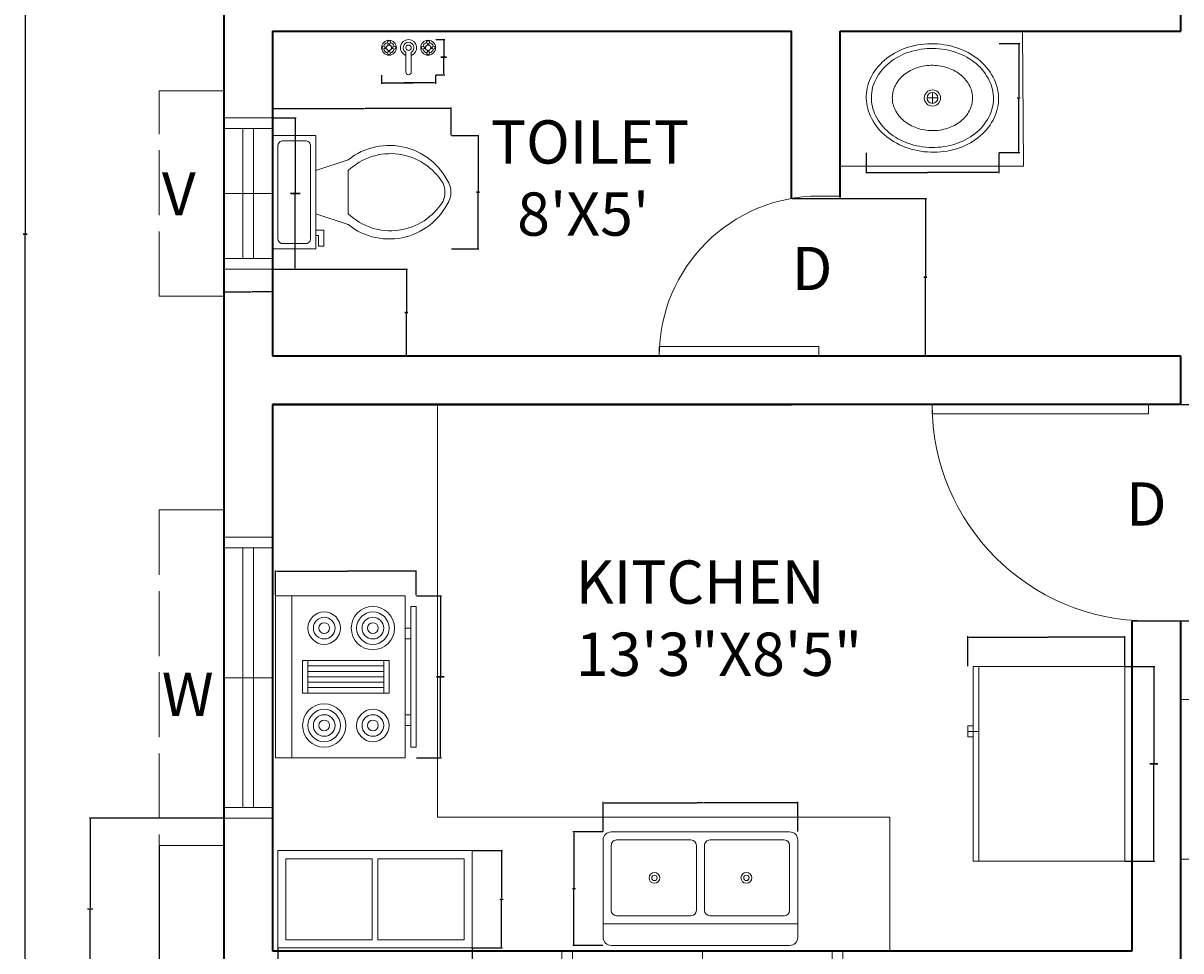
# Model space of a CAD drawing. Units: inches. Extents: x -35 to 832, y -515 to 219.
# Tile 3 of 7: x -35 to 179, y -163 to 9. Entities that reach past the tile are written whole.
import ezdxf

# ---------------------------------------------------------------- set-up
doc = ezdxf.new("R2010")
doc.units = ezdxf.units.IN
doc.header["$MEASUREMENT"] = 0
doc.linetypes.add('ACAD_ISO02W100', pattern=[15, 12, -3])
for name, color, linetype, lineweight in [('A-ANNO-TEXT', 7, 'Continuous', 18), ('A-AREA-IDEN', 7, 'Continuous', 18), ('A-DOOR', 4, 'Continuous', 18), ('A-EQPM', 8, 'Continuous', 18), ('A-FLOR-CASE', 3, 'Continuous', 18), ('A-FLOR-FIXT', 9, 'Continuous', 18), ('A-GLAZ', 2, 'Continuous', 18), ('A-GLAZ-OVHD', 2, 'ACAD_ISO02W100', 13), ('A-WALL', 10, 'Continuous', 35), ('S-ANNO-DIMS', 2, 'Continuous', 18)]:
    doc.layers.add(name, color=color, linetype=linetype, lineweight=lineweight)
doc.styles.get("Standard").update_dxf_attribs({"font": 'arial.ttf'})
doc.dimstyles.get("Standard").update_dxf_attribs({"dimtxt": 0.18, "dimasz": 0.18, "dimexe": 0.18, "dimexo": 0.0625, "dimgap": 0.09, "dimtad": 0, "dimtih": 1, "dimtoh": 1, "dimdec": 1, "dimzin": 0, "dimdsep": 46, "dimlunit": 4, "dimtxsty": 'Standard', "dimcen": 0.09, "dimclrd": 211, "dimclre": 4, "dimclrt": 3, "dimadec": 0, "dimazin": 0, "dimtfac": 0.5, "dimtdec": 1, "dimtofl": 0, "dimtmove": 0, "dimatfit": 3, "dimfxl": 1, "dimtfill": 2, "dimtfillclr": 61, "dimtolj": 1, "dimtzin": 0, "dimarcsym": 0})

# ---------------------------------------------------------------- blocks, each defined once
blk = doc.blocks.new('*U2')
for p, q in [((0, 0), (0, -6)), ((-40, 0), (-40, -6))]:
    blk.add_line(p, q)
blk.add_lwpolyline([(0, 0), (0, 40), (-1.75, 40), (-1.75, 0)], close=True)
blk.add_arc((0, 0), 40, 90, 180)
blk = doc.blocks.new('*U4')
for p, q in [((0, 0), (0, -100)), ((750, 0), (750, -100))]:
    blk.add_line(p, q)
blk.add_lwpolyline([(0, 0), (0, 750), (43.75, 750), (43.75, 0)], close=True)
blk.add_arc((0, 0), 750, 0, 90)
blk = doc.blocks.new('Range-Oven - 30 in top')
for p, q in [((0, -3), (30, -3)), ((12, -6), (18, -6)), ((13, -20), (13, -6)), ((14, -6), (14, -20)), ((15, -20), (15, -6)), ((16, -6), (16, -20)), ((17, -20), (17, -6)), ((18, -20), (12, -20)), ((6, -24), (6, -25)), ((8, -25), (8, -24)), ((22, -25), (22, -24)), ((24, -24), (24, -25))]:
    blk.add_line(p, q)
for points in [[(0, -24), (0, 0), (30, 0), (30, -24)], [(12, -21), (12, -5), (18, -5), (18, -21)], [(2, -26), (2, -25), (28, -25), (28, -26)]]:
    blk.add_lwpolyline(points, close=True)
for centre, radius in [((6, -9), 4), ((6, -9), 3), ((24, -9), 3), ((6, -9), 2), ((6, -9), 1), ((24, -9), 2), ((24, -9), 1), ((24, -18), 4), ((6, -18), 3), ((6, -18), 2), ((6, -18), 1), ((24, -18), 3), ((24, -18), 2), ((24, -18), 1)]:
    blk.add_circle(centre, radius)
blk = doc.blocks.new('Sink-double - 36 in top')
for p, q in [((-18, -4), (18, -4)), ((-0.75, -18.5), (-0.75, -6.5)), ((0.75, -6.5), (0.75, -18.5))]:
    blk.add_line(p, q)
for points in [[(-16.5, 0), (16.5, 0)], [(-18, -19.5), (-18, -1.5)], [(18, -1.5), (18, -19.5)], [(-15.5, -5.5), (-1.75, -5.5)], [(1.75, -5.5), (15.5, -5.5)], [(-16.5, -18.5), (-16.5, -6.5)], [(16.5, -6.5), (16.5, -18.5)], [(16.5, -21), (-16.5, -21)], [(-1.75, -19.5), (-15.5, -19.5)], [(15.5, -19.5), (1.75, -19.5)]]:
    blk.add_lwpolyline(points)
for centre, radius in [((-8.5, -12.5), 1), ((-8.5, -12.5), 0.5), ((8.5, -12.5), 1), ((8.5, -12.5), 0.5)]:
    blk.add_circle(centre, radius)
for centre, radius, start, end in [((-16.5, -1.5), 1.5, 90, 180), ((16.5, -1.5), 1.5, 0, 90), ((-15.5, -6.5), 1, 90, 180), ((-1.75, -6.5), 1, 0, 90), ((1.75, -6.5), 1, 90, 180), ((15.5, -6.5), 1, 0, 90), ((-15.5, -18.5), 1, 180, 270), ((-1.75, -18.5), 1, 270, 0), ((1.75, -18.5), 1, 180, 270), ((15.5, -18.5), 1, 270, 0), ((-16.5, -19.5), 1.5, 180, 270), ((16.5, -19.5), 1.5, 270, 0)]:
    blk.add_arc(centre, radius, start, end)
blk = doc.blocks.new('Refrigerator-2 door - 36 in top')
for p, q in [((0, -26.999999), (36, -26.999999)), ((12, -26.999999), (12, -28.999999)), ((11, -27.999999), (11, -28.999999)), ((11, -28.999999), (13, -28.999999)), ((13, -28.999999), (13, -27.999999))]:
    blk.add_line(p, q)
blk.add_lwpolyline([(0, -27.999999), (0, 0), (36, 0), (36, -27.999999)], close=True)
blk = doc.blocks.new('Wall Cabinet - 18 x 36 in front')
for p, q in [((17.5, -1.5), (17.5, -16.5)), ((18.5, -16.5), (18.5, -1.5))]:
    blk.add_line(p, q)
blk.add_lwpolyline([(0, -18), (0, 0), (36, 0), (36, -18)], close=True)
for points in [[(17.5, -16.5), (1.5, -16.5), (1.5, -1.5), (17.5, -1.5)], [(18.5, -1.5), (34.5, -1.5), (34.5, -16.5), (18.5, -16.5)]]:
    blk.add_lwpolyline(points)
blk = doc.blocks.new('Toilet - top')
for p, q in [((9.5, -6), (9.5, -2)), ((-10, -8.5), (-8, -8.5)), ((-10, -9.5), (-10, -8.5)), ((-8, -8.5), (-8, -8)), ((-7, -8), (-7, -9.5)), ((-4, -8), (-6, -14)), ((4, -8), (6, -14)), ((-7, -9.5), (-10, -9.5)), ((4, -14), (-4, -14))]:
    blk.add_line(p, q)
blk.add_lwpolyline([(10.5, -8), (10.5, 0), (-10.5, 0), (-10.5, -8)], close=True)
for points in [[(-9.5, -2), (-9.5, -6)], [(8.5, -1), (-8.5, -1)], [(-8.5, -7), (8.5, -7)]]:
    blk.add_lwpolyline(points)
for centre, radius, start, end in [((-8.62, -1.88), 0.884, 81.8699, 188.1301), ((8.62, -1.88), 0.884, 351.8699, 98.1301), ((-8.62, -6.12), 0.884, 171.8699, 278.1301), ((8.62, -6.12), 0.884, 261.8699, 8.1301), ((3.52, -21.58), 12.17, 141.4691, 247.9714), ((4.2, -21.82), 11.33, 136.3677, 238.9468), ((-3.52, -21.58), 12.17, 292.0284, 38.5307), ((-4.2, -21.82), 11.33, 301.053, 43.6321), ((0, -27.88), 4, 245.7318, 294.2682), ((0, -29), 4, 254.8605, 285.1395)]:
    blk.add_arc(centre, radius, start, end)
blk = doc.blocks.new('Sink - Oval top')
for p, q in [((-1, 0), (1, 0)), ((0, 1), (0, -1))]:
    blk.add_line(p, q)
for points in [[(-12.23, 0.39, 0.117634), (-11.46, -3.36, 0.104469), (-8.88, -6.8, 0.090016), (-5.08, -9.07, 0.08192), (-0.32, -10.02, 0.08192), (4.49, -9.38, 0.090016), (8.42, -7.36, 0.104469), (11.22, -4.09, 0.117634), (12.23, -0.39, 0.117634), (11.46, 3.36, 0.104469), (8.88, 6.8, 0.090016), (5.08, 9.07, 0.08192), (0.32, 10.02, 0.08192), (-4.49, 9.38, 0.090016), (-8.42, 7.36, 0.104469), (-11.22, 4.09, 0.117634)], [(-11.29, 0.16, 0.118622), (-10.52, -3.25, 0.104678), (-8.07, -6.36, 0.089562), (-4.54, -8.37, 0.081185), (-0.13, -9.15, 0.081185), (4.3, -8.49, 0.089562), (7.89, -6.58, 0.104678), (10.42, -3.55, 0.118622), (11.29, -0.16, 0.118622), (10.52, 3.25, 0.104678), (8.07, 6.36, 0.089562), (4.54, 8.37, 0.081185), (0.13, 9.15, 0.081185), (-4.3, 8.49, 0.089562), (-7.89, 6.58, 0.104678), (-10.42, 3.55, 0.118622)], [(-7.42, 0.08, 0.118283), (-6.91, -2.17, 0.104607), (-5.29, -4.21, 0.089718), (-2.97, -5.53, 0.081436), (-0.07, -6.04, 0.081436), (2.84, -5.59, 0.089718), (5.2, -4.33, 0.104607), (6.86, -2.32, 0.118283), (7.42, -0.08, 0.118283), (6.91, 2.17, 0.104607), (5.29, 4.21, 0.089718), (2.97, 5.53, 0.081436), (0.07, 6.04, 0.081436), (-2.84, 5.59, 0.089718), (-5.2, 4.33, 0.104607), (-6.86, 2.32, 0.118283)]]:
    blk.add_lwpolyline(points, format="xyb", close=True)
for radius in [1.5, 1]:
    blk.add_circle((0, 0), radius)
blk = doc.blocks.new('Faucet - Bathroom top')
for p, q in [((-4.107, 0.125), (-4.375, 0.125)), ((-3.75, 0.4788), (-3.75, 0.75)), ((-3.5, 0.482), (-3.5, 0.75)), ((-3.1461, 0.125), (-2.875, 0.125)), ((3.143, 0.125), (2.875, 0.125)), ((3.5, 0.4788), (3.5, 0.75)), ((3.75, 0.482), (3.75, 0.75)), ((4.1039, 0.125), (4.375, 0.125)), ((-4.1039, -0.125), (-4.375, -0.125)), ((-3.75, -0.4821), (-3.75, -0.75)), ((-3.5, -0.4789), (-3.5, -0.75)), ((-3.143, -0.125), (-2.875, -0.125)), ((-0.5, -0.8639), (-0.5, -4.5)), ((0.5, -4.5), (0.5, -0.8631)), ((3.1461, -0.125), (2.875, -0.125)), ((3.5, -0.4821), (3.5, -0.75)), ((3.75, -0.4789), (3.75, -0.75)), ((4.107, -0.125), (4.375, -0.125))]:
    blk.add_line(p, q)
for centre, radius in [((-3.625, 0), 1.375), ((-4.625, 0), 0.2795), ((-3.625, 0), 0.5), ((-3.625, 1), 0.2795), ((-2.625, 0), 0.2795), ((0, 0), 0.5), ((3.625, 0), 1.375), ((2.625, 0), 0.2795), ((3.625, 0), 0.5), ((3.625, 1), 0.2795), ((4.625, 0), 0.2795), ((-3.625, -1), 0.2795), ((3.625, -1), 0.2795)]:
    blk.add_circle(centre, radius)
for centre, radius, start, end in [((-3.625, 0), 1, 105.2407, 164.2093), ((-3.625, 0), 1, 16.44125, 74.07887), ((0, 0), 1.5, 289.6514, 250.3603), ((0, 0), 1, 300.3431, 239.7554), ((3.625, 0), 1, 106.12, 164.0884), ((3.625, 0), 1, 16.23422, 73.90469), ((-3.625, 0), 1, 196.2342, 253.9047), ((-3.625, 0), 1, 286.12, 344.0884), ((3.625, 0), 1, 196.4413, 254.0789), ((3.625, 0), 1, 285.2407, 344.2093), ((0, -4.5), 0.5, 180, 0)]:
    blk.add_arc(centre, radius, start, end)
blk = doc.blocks.new('WIN-48')
for p, q in [((0, 9), (0, 0)), ((2, 9), (2, 0)), ((26, 9), (26, 0)), ((50, 9), (50, 0)), ((52, 9), (52, 0)), ((2, 5.5), (50, 5.5)), ((2, 3.5), (50, 3.5))]:
    blk.add_line(p, q)
blk = doc.blocks.new('VENT-24')
for p, q in [((9, 28), (0, 28)), ((9, 26), (0, 26)), ((3.5, 26), (3.5, 2)), ((5.5, 26), (5.5, 2)), ((9, 14), (0, 14)), ((9, 2), (0, 2)), ((9, 0), (0, 0))]:
    blk.add_line(p, q)
blk = doc.blocks.new('WIN-48-HOOD')
for p, q in [((5, 12), (0, 12)), ((0, 12), (0, 0)), ((57, 12), (62, 12)), ((62, 12), (62, 0)), ((0, 0), (62, 0))]:
    blk.add_line(p, q)
blk = doc.blocks.new('VENT-24-HOOD')
for p, q in [((12, 38), (0, 38)), ((0, 0), (0, 38)), ((12, 33), (12, 38)), ((12, 5), (12, 0)), ((12, 0), (0, 0))]:
    blk.add_line(p, q)
blk = doc.blocks.new('*D65')
at = {"layer": 'Defpoints', "color": 0, "transparency": 16777216}
for p in [(10.8, -8.95), (15, -8.95), (10.8, -36.95)]:
    blk.add_point(p, dxfattribs=at)
at = {"layer": 'S-ANNO-DIMS', "color": 4, "lineweight": -2, "transparency": 16777216}
for p, q in [((10.86, -8.95), (15.18, -8.95)), ((10.86, -36.95), (15.18, -36.95))]:
    blk.add_line(p, q, dxfattribs=at)
at = {"layer": 'S-ANNO-DIMS', "color": 211, "lineweight": -2, "transparency": 16777216}
for p, q in [((15, -9.13), (15, -22.77)), ((15, -36.77), (15, -23.13))]:
    blk.add_line(p, q, dxfattribs=at)
at = {"layer": 'S-ANNO-DIMS', "color": 211, "transparency": 16777216}
for points in [[(14.97, -9.13), (15.03, -9.13), (15, -8.95)], [(14.97, -36.77), (15.03, -36.77), (15, -36.95)]]:
    blk.add_solid(points, dxfattribs=at)
at = {"layer": 'S-ANNO-DIMS', "color": 3, "transparency": 16777216, "insert": (15, -22.95), "char_height": 0.18, "attachment_point": 5, "bg_fill": 1, "box_fill_scale": 1.25, "bg_fill_color": 61, "bg_fill_transparency": 0}
blk.add_mtext('\\A1;VENT 2\'-4" TYP.', dxfattribs=at)
blk = doc.blocks.new('*D66')
at = {"layer": 'Defpoints', "color": 0, "transparency": 16777216}
for p in [(1.8, -36.95), (10.8, -36.95), (10.8, -41.15)]:
    blk.add_point(p, dxfattribs=at)
at = {"layer": 'S-ANNO-DIMS', "color": 4, "lineweight": -2, "transparency": 16777216}
for p, q in [((1.8, -37.01), (1.8, -41.33)), ((10.8, -37.01), (10.8, -41.33))]:
    blk.add_line(p, q, dxfattribs=at)
at = {"layer": 'S-ANNO-DIMS', "color": 211, "lineweight": -2, "transparency": 16777216}
for p, q in [((1.98, -41.15), (5.66, -41.15)), ((10.62, -41.15), (6.94, -41.15))]:
    blk.add_line(p, q, dxfattribs=at)
at = {"layer": 'S-ANNO-DIMS', "color": 211, "transparency": 16777216}
for points in [[(1.98, -41.12), (1.98, -41.18), (1.8, -41.15)], [(10.62, -41.12), (10.62, -41.18), (10.8, -41.15)]]:
    blk.add_solid(points, dxfattribs=at)
at = {"layer": 'S-ANNO-DIMS', "color": 3, "transparency": 16777216, "insert": (6.3, -41.15), "char_height": 0.18, "attachment_point": 5, "bg_fill": 1, "box_fill_scale": 1.25, "bg_fill_color": 61, "bg_fill_transparency": 0}
blk.add_mtext('\\A1;0\'-9" TYP.', dxfattribs=at)
blk = doc.blocks.new('*D75')
at = {"layer": 'Defpoints', "color": 0, "transparency": 16777216}
for p in [(37.35, -97.29), (41.85, -97.29), (37.35, -127.29)]:
    blk.add_point(p, dxfattribs=at)
at = {"layer": 'S-ANNO-DIMS', "color": 4, "lineweight": -2, "transparency": 16777216}
for p, q in [((37.41, -97.29), (42.03, -97.29)), ((37.41, -127.29), (42.03, -127.29))]:
    blk.add_line(p, q, dxfattribs=at)
at = {"layer": 'S-ANNO-DIMS', "color": 211, "lineweight": -2, "transparency": 16777216}
for p, q in [((41.85, -97.47), (41.85, -112.1)), ((41.85, -127.11), (41.85, -112.47))]:
    blk.add_line(p, q, dxfattribs=at)
at = {"layer": 'S-ANNO-DIMS', "color": 211, "transparency": 16777216}
for points in [[(41.82, -97.47), (41.88, -97.47), (41.85, -97.29)], [(41.82, -127.11), (41.88, -127.11), (41.85, -127.29)]]:
    blk.add_solid(points, dxfattribs=at)
at = {"layer": 'S-ANNO-DIMS', "color": 3, "transparency": 16777216, "insert": (41.85, -112.29), "char_height": 0.18, "attachment_point": 5, "bg_fill": 1, "box_fill_scale": 1.25, "bg_fill_color": 61, "bg_fill_transparency": 0}
blk.add_mtext('\\A1;RANGE 2\'-6"', dxfattribs=at)
blk = doc.blocks.new('*D76')
at = {"layer": 'Defpoints', "color": 0, "transparency": 16777216}
for p in [(11.35, -92.79), (11.35, -97.29), (37.35, -97.29)]:
    blk.add_point(p, dxfattribs=at)
at = {"layer": 'S-ANNO-DIMS', "color": 4, "lineweight": -2, "transparency": 16777216}
for p, q in [((11.35, -97.22), (11.35, -92.61)), ((37.35, -97.22), (37.35, -92.61))]:
    blk.add_line(p, q, dxfattribs=at)
at = {"layer": 'S-ANNO-DIMS', "color": 211, "lineweight": -2, "transparency": 16777216}
for p, q in [((11.53, -92.79), (24.02, -92.79)), ((37.17, -92.79), (24.68, -92.79))]:
    blk.add_line(p, q, dxfattribs=at)
at = {"layer": 'S-ANNO-DIMS', "color": 211, "transparency": 16777216}
for points in [[(11.53, -92.76), (11.53, -92.82), (11.35, -92.79)], [(37.17, -92.76), (37.17, -92.82), (37.35, -92.79)]]:
    blk.add_solid(points, dxfattribs=at)
at = {"layer": 'S-ANNO-DIMS', "color": 3, "transparency": 16777216, "insert": (24.35, -92.79), "char_height": 0.18, "attachment_point": 5, "bg_fill": 1, "box_fill_scale": 1.25, "bg_fill_color": 61, "bg_fill_transparency": 0}
blk.add_mtext('\\A1;2\'-2"', dxfattribs=at)
blk = doc.blocks.new('*D77')
at = {"layer": 'Defpoints', "color": 0, "transparency": 16777216}
for p in [(71.94, -135.56), (71.94, -140.96), (107.94, -140.96)]:
    blk.add_point(p, dxfattribs=at)
at = {"layer": 'S-ANNO-DIMS', "color": 4, "lineweight": -2, "transparency": 16777216}
for p, q in [((71.94, -140.9), (71.94, -135.38)), ((107.94, -140.9), (107.94, -135.38))]:
    blk.add_line(p, q, dxfattribs=at)
at = {"layer": 'S-ANNO-DIMS', "color": 211, "lineweight": -2, "transparency": 16777216}
for p, q in [((72.12, -135.56), (89.29, -135.56)), ((107.76, -135.56), (90.6, -135.56))]:
    blk.add_line(p, q, dxfattribs=at)
at = {"layer": 'S-ANNO-DIMS', "color": 211, "transparency": 16777216}
for points in [[(72.12, -135.53), (72.12, -135.59), (71.94, -135.56)], [(107.76, -135.53), (107.76, -135.59), (107.94, -135.56)]]:
    blk.add_solid(points, dxfattribs=at)
at = {"layer": 'S-ANNO-DIMS', "color": 3, "transparency": 16777216, "insert": (89.94, -135.56), "char_height": 0.18, "attachment_point": 5, "bg_fill": 1, "box_fill_scale": 1.25, "bg_fill_color": 61, "bg_fill_transparency": 0}
blk.add_mtext('\\A1;SINK 3\'-0"', dxfattribs=at)
blk = doc.blocks.new('*D78')
at = {"layer": 'Defpoints', "color": 0, "transparency": 16777216}
for p in [(71.94, -140.96), (66.54, -161.96), (71.94, -161.96)]:
    blk.add_point(p, dxfattribs=at)
at = {"layer": 'S-ANNO-DIMS', "color": 4, "lineweight": -2, "transparency": 16777216}
for p, q in [((71.88, -140.96), (66.36, -140.96)), ((71.88, -161.96), (66.36, -161.96))]:
    blk.add_line(p, q, dxfattribs=at)
at = {"layer": 'S-ANNO-DIMS', "color": 211, "lineweight": -2, "transparency": 16777216}
for p, q in [((66.54, -141.14), (66.54, -151.28)), ((66.54, -161.78), (66.54, -151.64))]:
    blk.add_line(p, q, dxfattribs=at)
at = {"layer": 'S-ANNO-DIMS', "color": 211, "transparency": 16777216}
for points in [[(66.51, -141.14), (66.57, -141.14), (66.54, -140.96)], [(66.51, -161.78), (66.57, -161.78), (66.54, -161.96)]]:
    blk.add_solid(points, dxfattribs=at)
at = {"layer": 'S-ANNO-DIMS', "color": 3, "transparency": 16777216, "insert": (66.54, -151.46), "char_height": 0.18, "attachment_point": 5, "bg_fill": 1, "box_fill_scale": 1.25, "bg_fill_color": 61, "bg_fill_transparency": 0}
blk.add_mtext('\\A1;1\'-9"', dxfattribs=at)
blk = doc.blocks.new('*D79')
at = {"layer": 'Defpoints', "color": 0, "transparency": 16777216}
for p in [(168.41, -110.38), (168.41, -146.38), (173.81, -146.38)]:
    blk.add_point(p, dxfattribs=at)
at = {"layer": 'S-ANNO-DIMS', "color": 4, "lineweight": -2, "transparency": 16777216}
for p, q in [((168.48, -110.38), (173.99, -110.38)), ((168.48, -146.38), (173.99, -146.38))]:
    blk.add_line(p, q, dxfattribs=at)
at = {"layer": 'S-ANNO-DIMS', "color": 211, "lineweight": -2, "transparency": 16777216}
for p, q in [((173.81, -110.56), (173.81, -128.19)), ((173.81, -146.2), (173.81, -128.56))]:
    blk.add_line(p, q, dxfattribs=at)
at = {"layer": 'S-ANNO-DIMS', "color": 211, "transparency": 16777216}
for points in [[(173.78, -110.56), (173.84, -110.56), (173.81, -110.38)], [(173.78, -146.2), (173.84, -146.2), (173.81, -146.38)]]:
    blk.add_solid(points, dxfattribs=at)
at = {"layer": 'S-ANNO-DIMS', "color": 3, "transparency": 16777216, "insert": (173.81, -128.38), "char_height": 0.18, "attachment_point": 5, "bg_fill": 1, "box_fill_scale": 1.25, "bg_fill_color": 61, "bg_fill_transparency": 0}
blk.add_mtext('\\A1;FRIDGE 3\'-0"', dxfattribs=at)
blk = doc.blocks.new('*D80')
at = {"layer": 'Defpoints', "color": 0, "transparency": 16777216}
for p in [(168.41, -104.98), (139.41, -110.38), (168.41, -110.38)]:
    blk.add_point(p, dxfattribs=at)
at = {"layer": 'S-ANNO-DIMS', "color": 4, "lineweight": -2, "transparency": 16777216}
for p, q in [((139.41, -110.31), (139.41, -104.8)), ((168.41, -110.31), (168.41, -104.8))]:
    blk.add_line(p, q, dxfattribs=at)
at = {"layer": 'S-ANNO-DIMS', "color": 211, "lineweight": -2, "transparency": 16777216}
for p, q in [((139.59, -104.98), (153.58, -104.98)), ((168.23, -104.98), (154.24, -104.98))]:
    blk.add_line(p, q, dxfattribs=at)
at = {"layer": 'S-ANNO-DIMS', "color": 211, "transparency": 16777216}
for points in [[(139.59, -104.95), (139.59, -105.01), (139.41, -104.98)], [(168.23, -104.95), (168.23, -105.01), (168.41, -104.98)]]:
    blk.add_solid(points, dxfattribs=at)
at = {"layer": 'S-ANNO-DIMS', "color": 3, "transparency": 16777216, "insert": (153.91, -104.98), "char_height": 0.18, "attachment_point": 5, "bg_fill": 1, "box_fill_scale": 1.25, "bg_fill_color": 61, "bg_fill_transparency": 0}
blk.add_mtext('\\A1;2\'-5"', dxfattribs=at)
blk = doc.blocks.new('*D81')
at = {"layer": 'Defpoints', "color": 0, "transparency": 16777216}
for p in [(11.74, -162.42), (47.74, -162.42), (47.74, -167.82)]:
    blk.add_point(p, dxfattribs=at)
at = {"layer": 'S-ANNO-DIMS', "color": 4, "lineweight": -2, "transparency": 16777216}
for p, q in [((11.74, -162.48), (11.74, -168)), ((47.74, -162.48), (47.74, -168))]:
    blk.add_line(p, q, dxfattribs=at)
at = {"layer": 'S-ANNO-DIMS', "color": 211, "lineweight": -2, "transparency": 16777216}
for p, q in [((11.92, -167.82), (28.83, -167.82)), ((47.56, -167.82), (30.65, -167.82))]:
    blk.add_line(p, q, dxfattribs=at)
at = {"layer": 'S-ANNO-DIMS', "color": 211, "transparency": 16777216}
for points in [[(11.92, -167.79), (11.92, -167.85), (11.74, -167.82)], [(47.56, -167.79), (47.56, -167.85), (47.74, -167.82)]]:
    blk.add_solid(points, dxfattribs=at)
at = {"layer": 'S-ANNO-DIMS', "color": 3, "transparency": 16777216, "insert": (29.74, -167.82), "char_height": 0.18, "attachment_point": 5, "bg_fill": 1, "box_fill_scale": 1.25, "bg_fill_color": 61, "bg_fill_transparency": 0}
blk.add_mtext('\\A1;CABINET 3\'-0"', dxfattribs=at)
blk = doc.blocks.new('*D82')
at = {"layer": 'Defpoints', "color": 0, "transparency": 16777216}
for p in [(47.74, -144.42), (53.14, -144.42), (47.74, -162.42)]:
    blk.add_point(p, dxfattribs=at)
at = {"layer": 'S-ANNO-DIMS', "color": 4, "lineweight": -2, "transparency": 16777216}
for p, q in [((47.8, -144.42), (53.32, -144.42)), ((47.8, -162.42), (53.32, -162.42))]:
    blk.add_line(p, q, dxfattribs=at)
at = {"layer": 'S-ANNO-DIMS', "color": 211, "lineweight": -2, "transparency": 16777216}
for p, q in [((53.14, -144.6), (53.14, -153.24)), ((53.14, -162.24), (53.14, -153.6))]:
    blk.add_line(p, q, dxfattribs=at)
at = {"layer": 'S-ANNO-DIMS', "color": 211, "transparency": 16777216}
for points in [[(53.11, -144.6), (53.17, -144.6), (53.14, -144.42)], [(53.11, -162.24), (53.17, -162.24), (53.14, -162.42)]]:
    blk.add_solid(points, dxfattribs=at)
at = {"layer": 'S-ANNO-DIMS', "color": 3, "transparency": 16777216, "insert": (53.14, -153.42), "char_height": 0.18, "attachment_point": 5, "bg_fill": 1, "box_fill_scale": 1.25, "bg_fill_color": 61, "bg_fill_transparency": 0}
blk.add_mtext('\\A1;1\'-6"', dxfattribs=at)
blk = doc.blocks.new('*D83')
at = {"layer": 'Defpoints', "color": 0, "transparency": 16777216}
for p in [(10.8, -7.24), (10.8, -12.2), (43.85, -12.2)]:
    blk.add_point(p, dxfattribs=at)
at = {"layer": 'S-ANNO-DIMS', "color": 4, "lineweight": -2, "transparency": 16777216}
for p, q in [((10.8, -12.13), (10.8, -7.06)), ((43.85, -12.13), (43.85, -7.06))]:
    blk.add_line(p, q, dxfattribs=at)
at = {"layer": 'S-ANNO-DIMS', "color": 211, "lineweight": -2, "transparency": 16777216}
for p, q in [((10.98, -7.24), (26.75, -7.24)), ((43.67, -7.24), (27.9, -7.24))]:
    blk.add_line(p, q, dxfattribs=at)
at = {"layer": 'S-ANNO-DIMS', "color": 211, "transparency": 16777216}
for points in [[(10.98, -7.21), (10.98, -7.27), (10.8, -7.24)], [(43.67, -7.21), (43.67, -7.27), (43.85, -7.24)]]:
    blk.add_solid(points, dxfattribs=at)
at = {"layer": 'S-ANNO-DIMS', "color": 3, "transparency": 16777216, "insert": (27.32, -7.24), "char_height": 0.18, "attachment_point": 5, "bg_fill": 1, "box_fill_scale": 1.25, "bg_fill_color": 61, "bg_fill_transparency": 0}
blk.add_mtext('\\A1;WC 2\'-9"', dxfattribs=at)
blk = doc.blocks.new('*D84')
at = {"layer": 'Defpoints', "color": 0, "transparency": 16777216}
for p in [(43.85, -12.2), (48.8, -12.2), (43.85, -33.2)]:
    blk.add_point(p, dxfattribs=at)
at = {"layer": 'S-ANNO-DIMS', "color": 4, "lineweight": -2, "transparency": 16777216}
for p, q in [((43.91, -12.2), (48.98, -12.2)), ((43.91, -33.2), (48.98, -33.2))]:
    blk.add_line(p, q, dxfattribs=at)
at = {"layer": 'S-ANNO-DIMS', "color": 211, "lineweight": -2, "transparency": 16777216}
for p, q in [((48.8, -12.38), (48.8, -22.51)), ((48.8, -33.02), (48.8, -22.88))]:
    blk.add_line(p, q, dxfattribs=at)
at = {"layer": 'S-ANNO-DIMS', "color": 211, "transparency": 16777216}
for points in [[(48.77, -12.38), (48.83, -12.38), (48.8, -12.2)], [(48.77, -33.02), (48.83, -33.02), (48.8, -33.2)]]:
    blk.add_solid(points, dxfattribs=at)
at = {"layer": 'S-ANNO-DIMS', "color": 3, "transparency": 16777216, "insert": (48.8, -22.7), "char_height": 0.18, "attachment_point": 5, "bg_fill": 1, "box_fill_scale": 1.25, "bg_fill_color": 61, "bg_fill_transparency": 0}
blk.add_mtext('\\A1;1\'-9"', dxfattribs=at)
blk = doc.blocks.new('*D85')
at = {"layer": 'Defpoints', "color": 0, "transparency": 16777216}
for p in [(120.58, -15.35), (145.13, -15.35), (145.13, -19.03)]:
    blk.add_point(p, dxfattribs=at)
at = {"layer": 'S-ANNO-DIMS', "color": 4, "lineweight": -2, "transparency": 16777216}
for p, q in [((120.58, -15.41), (120.58, -19.21)), ((145.13, -15.41), (145.13, -19.21))]:
    blk.add_line(p, q, dxfattribs=at)
at = {"layer": 'S-ANNO-DIMS', "color": 211, "lineweight": -2, "transparency": 16777216}
for p, q in [((120.76, -19.03), (131.91, -19.03)), ((144.95, -19.03), (133.8, -19.03))]:
    blk.add_line(p, q, dxfattribs=at)
at = {"layer": 'S-ANNO-DIMS', "color": 211, "transparency": 16777216}
for points in [[(120.76, -19), (120.76, -19.06), (120.58, -19.03)], [(144.95, -19), (144.95, -19.06), (145.13, -19.03)]]:
    blk.add_solid(points, dxfattribs=at)
at = {"layer": 'S-ANNO-DIMS', "color": 3, "transparency": 16777216, "insert": (132.85, -19.03), "char_height": 0.18, "attachment_point": 5, "bg_fill": 1, "box_fill_scale": 1.25, "bg_fill_color": 61, "bg_fill_transparency": 0}
blk.add_mtext('\\A1;BASIN 2\'-0 1/2"', dxfattribs=at)
blk = doc.blocks.new('*D86')
at = {"layer": 'Defpoints', "color": 0, "transparency": 16777216}
for p in [(145.13, 4.79), (148.81, 4.79), (145.13, -15.35)]:
    blk.add_point(p, dxfattribs=at)
at = {"layer": 'S-ANNO-DIMS', "color": 4, "lineweight": -2, "transparency": 16777216}
for p, q in [((145.19, 4.79), (148.99, 4.79)), ((145.19, -15.35), (148.99, -15.35))]:
    blk.add_line(p, q, dxfattribs=at)
at = {"layer": 'S-ANNO-DIMS', "color": 211, "lineweight": -2, "transparency": 16777216}
for p, q in [((148.81, 4.61), (148.81, -5.1)), ((148.81, -15.17), (148.81, -5.46))]:
    blk.add_line(p, q, dxfattribs=at)
at = {"layer": 'S-ANNO-DIMS', "color": 211, "transparency": 16777216}
for points in [[(148.78, 4.61), (148.84, 4.61), (148.81, 4.79)], [(148.78, -15.17), (148.84, -15.17), (148.81, -15.35)]]:
    blk.add_solid(points, dxfattribs=at)
at = {"layer": 'S-ANNO-DIMS', "color": 3, "transparency": 16777216, "insert": (148.81, -5.28), "char_height": 0.18, "attachment_point": 5, "bg_fill": 1, "box_fill_scale": 1.25, "bg_fill_color": 61, "bg_fill_transparency": 0}
blk.add_mtext('\\A1;1\'-8"', dxfattribs=at)
blk = doc.blocks.new('*D87')
at = {"layer": 'Defpoints', "color": 0, "transparency": 16777216}
for p in [(30.95, -0.99), (40.95, -0.99), (40.95, -2.49)]:
    blk.add_point(p, dxfattribs=at)
at = {"layer": 'S-ANNO-DIMS', "color": 4, "lineweight": -2, "transparency": 16777216}
for p, q in [((30.95, -1.05), (30.95, -2.67)), ((40.95, -1.05), (40.95, -2.67))]:
    blk.add_line(p, q, dxfattribs=at)
at = {"layer": 'S-ANNO-DIMS', "color": 211, "lineweight": -2, "transparency": 16777216}
for p, q in [((31.13, -2.49), (35.02, -2.49)), ((40.77, -2.49), (36.88, -2.49))]:
    blk.add_line(p, q, dxfattribs=at)
at = {"layer": 'S-ANNO-DIMS', "color": 211, "transparency": 16777216}
for points in [[(31.13, -2.46), (31.13, -2.52), (30.95, -2.49)], [(40.77, -2.46), (40.77, -2.52), (40.95, -2.49)]]:
    blk.add_solid(points, dxfattribs=at)
at = {"layer": 'S-ANNO-DIMS', "color": 3, "transparency": 16777216, "insert": (35.95, -2.49), "char_height": 0.18, "attachment_point": 5, "bg_fill": 1, "box_fill_scale": 1.25, "bg_fill_color": 61, "bg_fill_transparency": 0}
blk.add_mtext('\\A1;FAUCET 0\'-10"', dxfattribs=at)
blk = doc.blocks.new('*D88')
at = {"layer": 'Defpoints', "color": 0, "transparency": 16777216}
for p in [(40.95, 5.51), (42.45, 5.51), (40.95, -0.99)]:
    blk.add_point(p, dxfattribs=at)
at = {"layer": 'S-ANNO-DIMS', "color": 4, "lineweight": -2, "transparency": 16777216}
for p, q in [((41.02, 5.51), (42.63, 5.51)), ((41.02, -0.99), (42.63, -0.99))]:
    blk.add_line(p, q, dxfattribs=at)
at = {"layer": 'S-ANNO-DIMS', "color": 211, "lineweight": -2, "transparency": 16777216}
for p, q in [((42.45, 5.33), (42.45, 2.44)), ((42.45, -0.81), (42.45, 2.07))]:
    blk.add_line(p, q, dxfattribs=at)
at = {"layer": 'S-ANNO-DIMS', "color": 211, "transparency": 16777216}
for points in [[(42.42, 5.33), (42.48, 5.33), (42.45, 5.51)], [(42.42, -0.81), (42.48, -0.81), (42.45, -0.99)]]:
    blk.add_solid(points, dxfattribs=at)
at = {"layer": 'S-ANNO-DIMS', "color": 3, "transparency": 16777216, "insert": (42.45, 2.26), "char_height": 0.18, "attachment_point": 5, "bg_fill": 1, "box_fill_scale": 1.25, "bg_fill_color": 61, "bg_fill_transparency": 0}
blk.add_mtext('\\A1;0\'-6 1/2"', dxfattribs=at)
blk = doc.blocks.new('*D109')
at = {"layer": 'Defpoints', "color": 0, "transparency": 16777216}
for p in [(365.8, -100.95), (-10.2, -143.45), (365.8, -279.7)]:
    blk.add_point(p, dxfattribs=at)
at = {"layer": 'S-ANNO-DIMS', "color": 4, "lineweight": -2, "transparency": 16777216}
for p, q in [((365.8, -101.01), (365.8, -279.88)), ((-10.2, -143.51), (-10.2, -279.88))]:
    blk.add_line(p, q, dxfattribs=at)
at = {"layer": 'S-ANNO-DIMS', "color": 211, "lineweight": -2, "transparency": 16777216}
for p, q in [((-10.02, -279.7), (177.4, -279.7)), ((365.62, -279.7), (178.2, -279.7))]:
    blk.add_line(p, q, dxfattribs=at)
at = {"layer": 'S-ANNO-DIMS', "color": 211, "transparency": 16777216}
for points in [[(-10.02, -279.67), (-10.02, -279.73), (-10.2, -279.7)], [(365.62, -279.67), (365.62, -279.73), (365.8, -279.7)]]:
    blk.add_solid(points, dxfattribs=at)
at = {"layer": 'S-ANNO-DIMS', "color": 3, "transparency": 16777216, "insert": (177.8, -279.7), "char_height": 0.18, "attachment_point": 5, "bg_fill": 1, "box_fill_scale": 1.25, "bg_fill_color": 61, "bg_fill_transparency": 0}
blk.add_mtext('\\A1;31\'-4"', dxfattribs=at)
blk = doc.blocks.new('*D110')
at = {"layer": 'Defpoints', "color": 0, "transparency": 16777216}
for p in [(59.3, 194.05), (-34.95, -254.95), (129.8, -254.95)]:
    blk.add_point(p, dxfattribs=at)
at = {"layer": 'S-ANNO-DIMS', "color": 4, "lineweight": -2, "transparency": 16777216}
for p, q in [((59.24, 194.05), (-35.13, 194.05)), ((129.74, -254.95), (-35.13, -254.95))]:
    blk.add_line(p, q, dxfattribs=at)
at = {"layer": 'S-ANNO-DIMS', "color": 211, "lineweight": -2, "transparency": 16777216}
for p, q in [((-34.95, 193.87), (-34.95, -30.27)), ((-34.95, -254.77), (-34.95, -30.63))]:
    blk.add_line(p, q, dxfattribs=at)
at = {"layer": 'S-ANNO-DIMS', "color": 211, "transparency": 16777216}
for points in [[(-34.98, 193.87), (-34.92, 193.87), (-34.95, 194.05)], [(-34.98, -254.77), (-34.92, -254.77), (-34.95, -254.95)]]:
    blk.add_solid(points, dxfattribs=at)
at = {"layer": 'S-ANNO-DIMS', "color": 3, "transparency": 16777216, "insert": (-34.95, -30.45), "char_height": 0.18, "attachment_point": 5, "bg_fill": 1, "box_fill_scale": 1.25, "bg_fill_color": 61, "bg_fill_transparency": 0}
blk.add_mtext('\\A1;37\'-5"', dxfattribs=at)
blk = doc.blocks.new('*D113')
at = {"layer": 'Defpoints', "color": 0, "transparency": 16777216}
for p in [(106.8, -23.86), (106.8, -52.95), (131.55, -52.95)]:
    blk.add_point(p, dxfattribs=at)
at = {"layer": 'S-ANNO-DIMS', "color": 4, "lineweight": -2, "transparency": 16777216}
for p, q in [((106.86, -23.86), (131.73, -23.86)), ((106.86, -52.95), (131.73, -52.95))]:
    blk.add_line(p, q, dxfattribs=at)
at = {"layer": 'S-ANNO-DIMS', "color": 211, "lineweight": -2, "transparency": 16777216}
for p, q in [((131.55, -24.04), (131.55, -38.22)), ((131.55, -52.77), (131.55, -38.59))]:
    blk.add_line(p, q, dxfattribs=at)
at = {"layer": 'S-ANNO-DIMS', "color": 211, "transparency": 16777216}
for points in [[(131.52, -24.04), (131.58, -24.04), (131.55, -23.86)], [(131.52, -52.77), (131.58, -52.77), (131.55, -52.95)]]:
    blk.add_solid(points, dxfattribs=at)
at = {"layer": 'S-ANNO-DIMS', "color": 3, "transparency": 16777216, "insert": (131.55, -38.41), "char_height": 0.18, "attachment_point": 5, "bg_fill": 1, "box_fill_scale": 1.25, "bg_fill_color": 61, "bg_fill_transparency": 0}
blk.add_mtext('\\A1;2\'-5"', dxfattribs=at)
blk = doc.blocks.new('*D114')
at = {"layer": 'Defpoints', "color": 0, "transparency": 16777216}
for p in [(169.8, -61.95), (169.8, -101.95), (194.55, -101.95)]:
    blk.add_point(p, dxfattribs=at)
at = {"layer": 'S-ANNO-DIMS', "color": 4, "lineweight": -2, "transparency": 16777216}
for p, q in [((169.86, -61.95), (194.73, -61.95)), ((169.86, -101.95), (194.73, -101.95))]:
    blk.add_line(p, q, dxfattribs=at)
at = {"layer": 'S-ANNO-DIMS', "color": 211, "lineweight": -2, "transparency": 16777216}
for p, q in [((194.55, -62.13), (194.55, -81.77)), ((194.55, -101.77), (194.55, -82.13))]:
    blk.add_line(p, q, dxfattribs=at)
at = {"layer": 'S-ANNO-DIMS', "color": 211, "transparency": 16777216}
for points in [[(194.52, -62.13), (194.58, -62.13), (194.55, -61.95)], [(194.52, -101.77), (194.58, -101.77), (194.55, -101.95)]]:
    blk.add_solid(points, dxfattribs=at)
at = {"layer": 'S-ANNO-DIMS', "color": 3, "transparency": 16777216, "insert": (194.55, -81.95), "char_height": 0.18, "attachment_point": 5, "bg_fill": 1, "box_fill_scale": 1.25, "bg_fill_color": 61, "bg_fill_transparency": 0}
blk.add_mtext('\\A1;3\'-4"', dxfattribs=at)
blk = doc.blocks.new('*D116')
at = {"layer": 'Defpoints', "color": 0, "transparency": 16777216}
for p in [(-22.95, -138.45), (1.8, -138.45), (1.8, -171.95)]:
    blk.add_point(p, dxfattribs=at)
at = {"layer": 'S-ANNO-DIMS', "color": 4, "lineweight": -2, "transparency": 16777216}
for p, q in [((1.74, -138.45), (-23.13, -138.45)), ((1.74, -171.95), (-23.13, -171.95))]:
    blk.add_line(p, q, dxfattribs=at)
at = {"layer": 'S-ANNO-DIMS', "color": 211, "lineweight": -2, "transparency": 16777216}
for p, q in [((-22.95, -138.63), (-22.95, -155.02)), ((-22.95, -171.77), (-22.95, -155.38))]:
    blk.add_line(p, q, dxfattribs=at)
at = {"layer": 'S-ANNO-DIMS', "color": 211, "transparency": 16777216}
for points in [[(-22.98, -138.63), (-22.92, -138.63), (-22.95, -138.45)], [(-22.98, -171.77), (-22.92, -171.77), (-22.95, -171.95)]]:
    blk.add_solid(points, dxfattribs=at)
at = {"layer": 'S-ANNO-DIMS', "color": 3, "transparency": 16777216, "insert": (-22.95, -155.2), "char_height": 0.18, "attachment_point": 5, "bg_fill": 1, "box_fill_scale": 1.25, "bg_fill_color": 61, "bg_fill_transparency": 0}
blk.add_mtext('\\A1;2\'-9 1/2"', dxfattribs=at)
blk = doc.blocks.new('*D117')
at = {"layer": 'Defpoints', "color": 0, "transparency": 16777216}
for p in [(10.8, -36.95), (10.8, -52.95), (35.55, -52.95)]:
    blk.add_point(p, dxfattribs=at)
at = {"layer": 'S-ANNO-DIMS', "color": 4, "lineweight": -2, "transparency": 16777216}
for p, q in [((10.86, -36.95), (35.73, -36.95)), ((10.86, -52.95), (35.73, -52.95))]:
    blk.add_line(p, q, dxfattribs=at)
at = {"layer": 'S-ANNO-DIMS', "color": 211, "lineweight": -2, "transparency": 16777216}
for p, q in [((35.55, -37.13), (35.55, -44.77)), ((35.55, -52.77), (35.55, -45.13))]:
    blk.add_line(p, q, dxfattribs=at)
at = {"layer": 'S-ANNO-DIMS', "color": 211, "transparency": 16777216}
for points in [[(35.52, -37.13), (35.58, -37.13), (35.55, -36.95)], [(35.52, -52.77), (35.58, -52.77), (35.55, -52.95)]]:
    blk.add_solid(points, dxfattribs=at)
at = {"layer": 'S-ANNO-DIMS', "color": 3, "transparency": 16777216, "insert": (35.55, -44.95), "char_height": 0.18, "attachment_point": 5, "bg_fill": 1, "box_fill_scale": 1.25, "bg_fill_color": 61, "bg_fill_transparency": 0}
blk.add_mtext('\\A1;1\'-4"', dxfattribs=at)

msp = doc.modelspace()

# ---------------------------------------------------------------- linework, layer by layer
at = {"layer": 'A-FLOR-CASE'}
for p, q in [((149.69, -17.88), (149.5, 7.05)), ((115.8, -17.88), (149.69, -17.88)), ((41.33, -61.95), (41.33, -138.22)), ((41.33, -138.22), (124.99, -138.22)), ((124.99, -138.22), (124.99, -162.95))]:
    msp.add_line(p, q, dxfattribs=at)
at = {"layer": 'A-WALL'}
for p, q in [((1.8, 182.05), (1.8, 7.05)), ((178.8, 7.05), (178.8, 16.05)), ((1.8, 7.05), (1.8, -52.95)), ((10.8, 7.05), (106.8, 7.05)), ((10.8, 7.05), (10.8, -52.95)), ((106.8, -23.86), (106.8, 7.05)), ((115.8, 7.05), (178.8, 7.05)), ((115.8, -23.69), (115.8, 7.05)), ((1.8, -52.95), (1.8, -171.95)), ((10.8, -52.95), (106.8, -52.95)), ((106.8, -52.95), (115.8, -52.95)), ((115.8, -52.95), (178.8, -52.95)), ((178.8, -61.95), (178.8, -52.95)), ((10.8, -61.95), (106.8, -61.95)), ((10.8, -61.95), (10.8, -162.95)), ((178.8, -61.95), (10.8, -61.95)), ((169.8, -62.06), (169.8, -61.95)), ((169.8, -162.95), (169.8, -101.95)), ((178.8, -171.95), (178.8, -101.95)), ((10.8, -162.95), (169.8, -162.95))]:
    msp.add_line(p, q, dxfattribs=at)

# ---------------------------------------------------------------- block references
at = {"layer": 'A-DOOR', "xscale": 0.0393700787401575, "yscale": 0.0393700787401575, "zscale": 0.0393700787401575, "rotation": 90}
msp.add_blockref('*U4', (111.86, -52.95), dxfattribs=at)
at = {"layer": 'A-DOOR', "rotation": 90}
msp.add_blockref('*U2', (172.8, -61.95), dxfattribs=at)
at = {"layer": 'A-DOOR', "xscale": 0.0393700787401575, "yscale": 0.0393700787401575, "zscale": 0.0393700787401575}
msp.add_blockref('*U4', (178.8, -146.01), dxfattribs=at)
at = {"layer": 'A-EQPM'}
for name, p, rotation in [('Range-Oven - 30 in top', (11.35, -127.29), 90), ('Refrigerator-2 door - 36 in top', (168.41, -110.38), 270)]:
    msp.add_blockref(name, p, dxfattribs=dict(at, rotation=rotation))
at = {"layer": 'A-FLOR-CASE'}
msp.add_blockref('Wall Cabinet - 18 x 36 in front', (11.74, -144.42), dxfattribs=at)
at = {"layer": 'A-FLOR-FIXT'}
for name, p in [('Faucet - Bathroom top', (35.95, 4.01)), ('Sink - Oval top', (132.85, -5.28))]:
    msp.add_blockref(name, p, dxfattribs=at)
for name, p, rotation in [('Toilet - top', (10.8, -22.7), 90), ('Sink-double - 36 in top', (89.94, -161.96), 180)]:
    msp.add_blockref(name, p, dxfattribs=dict(at, rotation=rotation))
at = {"layer": 'A-GLAZ'}
for name, p in [('VENT-24', (1.8, -36.95)), ('WIN-48', (64.3, -171.95))]:
    msp.add_blockref(name, p, dxfattribs=at)
at = {"layer": 'A-GLAZ', "rotation": 90.00000000000003}
msp.add_blockref('WIN-48', (10.8, -138.45), dxfattribs=at)
at = {"layer": 'A-GLAZ-OVHD'}
msp.add_blockref('VENT-24-HOOD', (-10.2, -41.95), dxfattribs=at)
at = {"layer": 'A-GLAZ-OVHD', "rotation": 270}
msp.add_blockref('WIN-48-HOOD', (-10.2, -81.45), dxfattribs=at)

# ---------------------------------------------------------------- texts
at = {"layer": 'A-ANNO-TEXT'}
for s, p in [('V', (-9.69, -27)), ('D', (106.84, -40.81)), ('D', (168.65, -84.34)), ('W', (-9.69, -119.52))]:
    msp.add_text(s, height=8, dxfattribs=at).set_placement(p)
at = {"layer": 'A-AREA-IDEN', "char_height": 8, "attachment_point": 1}
for s, insert in [("TOILET\\P  8'X5'", (51.15, -9.41)), ('KITCHEN\\P13\'3"X8\'5"', (66.87, -90.78))]:
    msp.add_mtext_dynamic_manual_height_columns(s, width=50.3004, gutter_width=1, heights=[0], dxfattribs=dict(at, insert=insert))

# ---------------------------------------------------------------- dimensions: what is measured, and where the dimension line sits
at = {"layer": 'S-ANNO-DIMS'}
for base, p1, p2, angle, picture, middle in [((-34.95, -254.95), (59.3, 194.05), (129.8, -254.95), 90, '*D110', (-34.95, -30.45)), ((42.45, 5.51), (40.95, -0.99), (40.95, 5.51), 90, '*D88', (42.45, 2.26)), ((148.81, 4.79), (145.13, -15.35), (145.13, 4.79), 90, '*D86', (148.81, -5.28)), ((48.8, -12.2), (43.85, -33.2), (43.85, -12.2), 90, '*D84', (48.8, -22.7)), ((131.55, -52.95), (106.8, -23.86), (106.8, -52.95), 270, '*D113', (131.55, -38.41)), ((35.55, -52.95), (10.8, -36.95), (10.8, -52.95), 270, '*D117', (35.55, -44.95)), ((194.55, -101.95), (169.8, -61.95), (169.8, -101.95), 270, '*D114', (194.55, -81.95)), ((11.35, -92.79), (37.35, -97.29), (11.35, -97.29), 180, '*D76', (24.35, -92.79)), ((-22.95, -138.45), (1.8, -171.95), (1.8, -138.45), 90, '*D116', (-22.95, -155.2)), ((66.54, -161.96), (71.94, -140.96), (71.94, -161.96), 270, '*D78', (66.54, -151.46)), ((53.14, -144.42), (47.74, -162.42), (47.74, -144.42), 90, '*D82', (53.14, -153.42))]:
    dim = msp.add_linear_dim(base=base, p1=p1, p2=p2, angle=angle, dimstyle='Standard', override={"dimdec": 1, "dimlfac": 1, "dimrnd": 0, "dimzin": 1, "dimdsep": 46, "dimlunit": 4, "dimfrac": 2}, dxfattribs=at)
    dim.commit()
    dim.dimension.update_dxf_attribs({"geometry": picture, "text_midpoint": middle})
for base, p1, p2, text, picture, middle in [((40.95, -2.49), (30.95, -0.99), (40.95, -0.99), 'FAUCET <>', '*D87', (35.95, -2.49)), ((145.1293, -19.0334), (120.5784, -15.3507), (145.1293, -15.3507), 'BASIN <>', '*D85', (132.8538, -19.0334)), ((10.8, -41.15), (1.8, -36.95), (10.8, -36.95), '<> TYP.', '*D66', (6.3, -41.15)), ((47.74, -167.82), (11.74, -162.42), (47.74, -162.42), 'CABINET <>', '*D81', (29.74, -167.82))]:
    dim = msp.add_linear_dim(base=base, p1=p1, p2=p2, text=text, dimstyle='Standard', override={"dimdec": 1, "dimlfac": 1, "dimrnd": 0, "dimzin": 1, "dimdsep": 46, "dimlunit": 4, "dimfrac": 2}, dxfattribs=at)
    dim.commit()
    dim.dimension.update_dxf_attribs({"geometry": picture, "text_midpoint": middle})
for base, p1, p2, angle, text, picture, middle in [((10.8006, -7.2397), (43.8469, -12.1967), (10.8006, -12.1967), 180, 'WC <>', '*D83', (27.3238, -7.2397)), ((15, -8.95), (10.8, -36.95), (10.8, -8.95), 90, 'VENT <> TYP.', '*D65', (15, -22.95)), ((41.85, -97.29), (37.35, -127.29), (37.35, -97.29), 90, 'RANGE <>', '*D75', (41.85, -112.29)), ((173.81, -146.38), (168.41, -110.38), (168.41, -146.38), 270, 'FRIDGE <>', '*D79', (173.81, -128.38)), ((71.94, -135.56), (107.94, -140.96), (71.94, -140.96), 180, 'SINK <>', '*D77', (89.94, -135.56))]:
    dim = msp.add_linear_dim(base=base, p1=p1, p2=p2, angle=angle, text=text, dimstyle='Standard', override={"dimdec": 1, "dimlfac": 1, "dimrnd": 0, "dimzin": 1, "dimdsep": 46, "dimlunit": 4, "dimfrac": 2}, dxfattribs=at)
    dim.commit()
    dim.dimension.update_dxf_attribs({"geometry": picture, "text_midpoint": middle})
for base, p1, p2, picture, middle in [((365.8, -279.7), (-10.2, -143.45), (365.8, -100.95), '*D109', (177.8, -279.7)), ((168.41, -104.98), (139.41, -110.38), (168.41, -110.38), '*D80', (153.91, -104.98))]:
    dim = msp.add_linear_dim(base=base, p1=p1, p2=p2, dimstyle='Standard', override={"dimdec": 1, "dimlfac": 1, "dimrnd": 0, "dimzin": 1, "dimdsep": 46, "dimlunit": 4, "dimfrac": 2}, dxfattribs=at)
    dim.commit()
    dim.dimension.update_dxf_attribs({"geometry": picture, "text_midpoint": middle})

doc.saveas('drawing.dxf')
